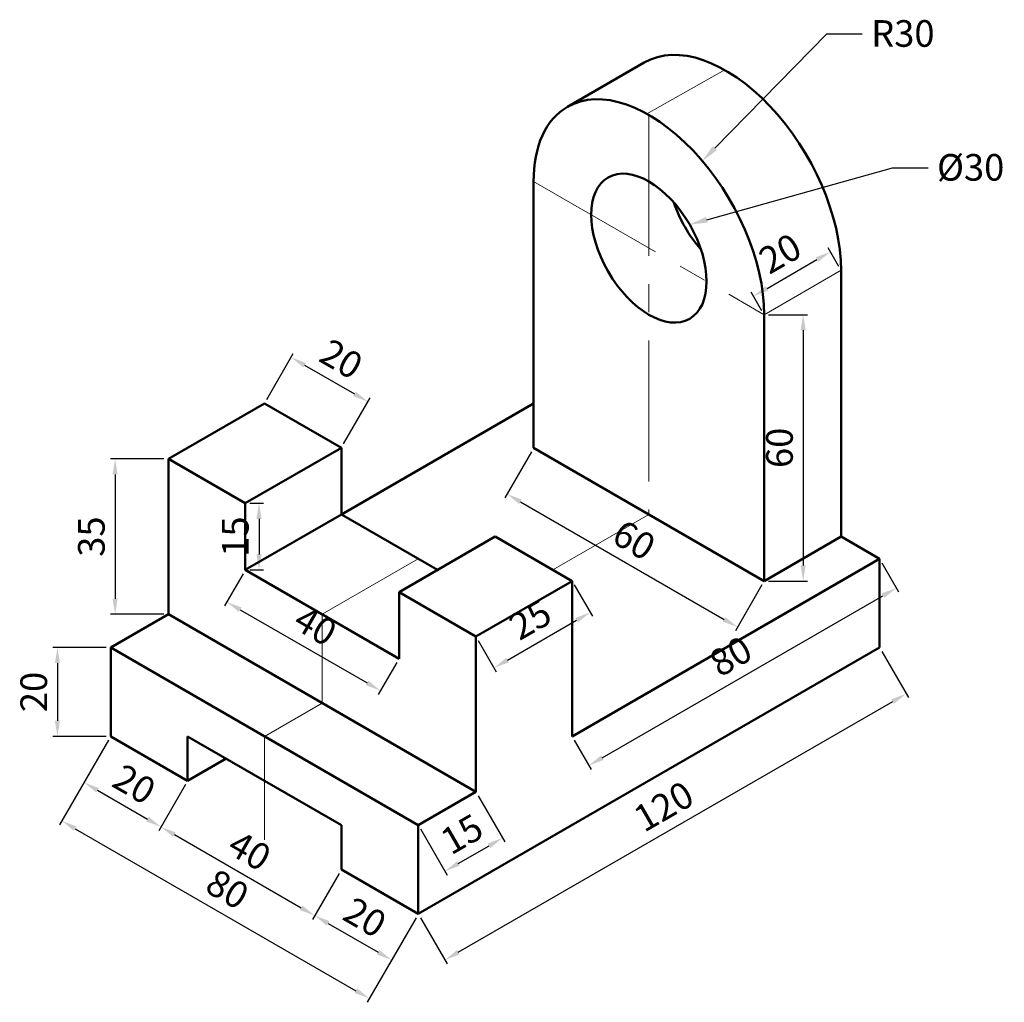
# Model space of a CAD drawing. Units: millimetres. Extents: x 3098 to 3319, y 970 to 1192.
import ezdxf
from ezdxf import colors
from ezdxf.entities.mleader import LeaderData, LeaderLine
from ezdxf.math import Vec2, Vec3

# ---------------------------------------------------------------- set-up
doc = ezdxf.new("R2010")
doc.units = ezdxf.units.MM
doc.linetypes.add('CENTER', pattern=[50.8, 31.75, -6.35, 6.35, -6.35])
for name, color, linetype, lineweight in [('M-CNTR', 1, 'CENTER', 18), ('M-DIMS', 3, 'Continuous', 25), ('M-OUTL', 7, 'Continuous', 50)]:
    doc.layers.add(name, color=color, linetype=linetype, lineweight=lineweight)
doc.styles.get("Standard").update_dxf_attribs({"font": 'arial.ttf'})
doc.dimstyles.new('AM_ISO$0', dxfattribs={"dimtxt": 6, "dimasz": 3.5, "dimexe": 1, "dimexo": 1, "dimgap": 1.5, "dimtad": 1, "dimdsep": 46, "dimtxsty": 'Standard', "dimcen": 0, "dimclrd": 256, "dimclre": 256, "dimclrt": 2, "dimadec": 0, "dimazin": 2, "dimtp": 0.1, "dimtm": 0.1, "dimtfac": 0.71, "dimtmove": 0, "dimatfit": 3, "dimfxl": 1, "dimlwd": -1, "dimlwe": -1, "dimarcsym": 1})

# ---------------------------------------------------------------- blocks, each defined once
blk = doc.blocks.new('*D3')
at = {"layer": 'Defpoints', "color": 0, "transparency": 16777216}
for p in [(3291.25, 1050.05), (3297.25, 1039.66), (3187.33, 990.05)]:
    blk.add_point(p, dxfattribs=at)
at = {"layer": 'M-DIMS', "color": 0, "linetype": 'ByBlock', "transparency": 16777216}
for p, q in [((3291.75, 1049.18), (3297.75, 1038.79)), ((3196.36, 981.41), (3294.22, 1037.91)), ((3187.83, 989.18), (3193.83, 978.79))]:
    blk.add_line(p, q, dxfattribs=at)
at = {"layer": 'M-DIMS', "color": 0, "transparency": 16777216}
for points in [[(3293.93, 1038.41), (3294.51, 1037.4), (3297.25, 1039.66)], [(3196.07, 981.91), (3196.65, 980.9), (3193.33, 979.66)]]:
    blk.add_solid(points, dxfattribs=at)
at = {"layer": 'M-DIMS', "color": 0, "transparency": 16777216, "insert": (3243.01, 1013.61), "char_height": 6, "attachment_point": 5, "rotation": 30}
blk.add_mtext('120', dxfattribs=at)
blk = doc.blocks.new('*D4')
at = {"layer": 'Defpoints', "color": 0, "transparency": 16777216}
for p in [(3291.25, 1070.05), (3295.05, 1063.48), (3221.97, 1030.05)]:
    blk.add_point(p, dxfattribs=at)
at = {"layer": 'M-DIMS', "color": 0, "linetype": 'ByBlock', "transparency": 16777216}
for p, q in [((3291.75, 1069.18), (3295.55, 1062.61)), ((3228.8, 1025.23), (3292.02, 1061.73)), ((3222.47, 1029.18), (3226.27, 1022.61))]:
    blk.add_line(p, q, dxfattribs=at)
at = {"layer": 'M-DIMS', "color": 0, "transparency": 16777216}
for points in [[(3291.72, 1062.24), (3292.31, 1061.23), (3295.05, 1063.48)], [(3228.5, 1025.74), (3229.09, 1024.73), (3225.77, 1023.48)]]:
    blk.add_solid(points, dxfattribs=at)
at = {"layer": 'M-DIMS', "color": 0, "transparency": 16777216, "insert": (3258.12, 1047.43), "char_height": 6, "attachment_point": 5, "rotation": 30}
blk.add_mtext('80', dxfattribs=at)
blk = doc.blocks.new('*D5')
at = {"layer": 'Defpoints', "color": 0, "transparency": 16777216}
for p in [(3221.97, 1065.05), (3226.06, 1057.98), (3200.32, 1052.55)]:
    blk.add_point(p, dxfattribs=at)
at = {"layer": 'M-DIMS', "color": 0, "linetype": 'ByBlock', "transparency": 16777216}
for p, q in [((3222.47, 1064.18), (3226.56, 1057.11)), ((3207.44, 1047.23), (3223.02, 1056.23)), ((3200.82, 1051.68), (3204.9, 1044.61))]:
    blk.add_line(p, q, dxfattribs=at)
at = {"layer": 'M-DIMS', "color": 0, "transparency": 16777216}
for points in [[(3222.73, 1056.73), (3223.32, 1055.72), (3226.06, 1057.98)], [(3207.14, 1047.73), (3207.73, 1046.72), (3204.4, 1045.48)]]:
    blk.add_solid(points, dxfattribs=at)
at = {"layer": 'M-DIMS', "color": 0, "transparency": 16777216, "insert": (3212.95, 1055.68), "char_height": 6, "attachment_point": 5, "rotation": 30}
blk.add_mtext('25', dxfattribs=at)
blk = doc.blocks.new('*D6')
at = {"layer": 'Defpoints', "color": 0, "transparency": 16777216}
for p in [(3131.04, 1092.55), (3119.04, 1057.55), (3131.04, 1057.55)]:
    blk.add_point(p, dxfattribs=at)
at = {"layer": 'M-DIMS', "color": 0, "linetype": 'ByBlock', "transparency": 16777216}
for p, q in [((3130.04, 1092.55), (3118.04, 1092.55)), ((3119.04, 1089.05), (3119.04, 1061.05)), ((3130.04, 1057.55), (3118.04, 1057.55))]:
    blk.add_line(p, q, dxfattribs=at)
at = {"layer": 'M-DIMS', "color": 0, "transparency": 16777216}
for points in [[(3118.46, 1089.05), (3119.62, 1089.05), (3119.04, 1092.55)], [(3118.46, 1061.05), (3119.62, 1061.05), (3119.04, 1057.55)]]:
    blk.add_solid(points, dxfattribs=at)
at = {"layer": 'M-DIMS', "color": 0, "transparency": 16777216, "insert": (3114.47, 1075.05), "char_height": 6, "attachment_point": 5, "rotation": 90}
blk.add_mtext('35', dxfattribs=at)
blk = doc.blocks.new('*D7')
at = {"layer": 'Defpoints', "color": 0, "transparency": 16777216}
for p in [(3118.05, 1050.05), (3106.05, 1030.05), (3118.05, 1030.05)]:
    blk.add_point(p, dxfattribs=at)
at = {"layer": 'M-DIMS', "color": 0, "linetype": 'ByBlock', "transparency": 16777216}
for p, q in [((3117.05, 1050.05), (3105.05, 1050.05)), ((3106.05, 1046.55), (3106.05, 1033.55)), ((3117.05, 1030.05), (3105.05, 1030.05))]:
    blk.add_line(p, q, dxfattribs=at)
at = {"layer": 'M-DIMS', "color": 0, "transparency": 16777216}
for points in [[(3105.47, 1046.55), (3106.63, 1046.55), (3106.05, 1050.05)], [(3105.47, 1033.55), (3106.63, 1033.55), (3106.05, 1030.05)]]:
    blk.add_solid(points, dxfattribs=at)
at = {"layer": 'M-DIMS', "color": 0, "transparency": 16777216, "insert": (3101.49, 1040.05), "char_height": 6, "attachment_point": 5, "rotation": 90}
blk.add_mtext('20', dxfattribs=at)
blk = doc.blocks.new('*D8')
at = {"layer": 'Defpoints', "color": 0, "transparency": 16777216}
for p in [(3118.05, 1030.05), (3135.37, 1020.05), (3129.37, 1009.66)]:
    blk.add_point(p, dxfattribs=at)
at = {"layer": 'M-DIMS', "color": 0, "linetype": 'ByBlock', "transparency": 16777216}
for p, q in [((3117.55, 1029.18), (3111.55, 1018.79)), ((3134.87, 1019.18), (3128.87, 1008.79)), ((3115.08, 1017.91), (3126.34, 1011.41))]:
    blk.add_line(p, q, dxfattribs=at)
at = {"layer": 'M-DIMS', "color": 0, "transparency": 16777216}
for points in [[(3115.37, 1018.41), (3114.79, 1017.4), (3112.05, 1019.66)], [(3126.63, 1011.91), (3126.05, 1010.9), (3129.37, 1009.66)]]:
    blk.add_solid(points, dxfattribs=at)
at = {"layer": 'M-DIMS', "color": 0, "transparency": 16777216, "insert": (3122.99, 1018.61), "char_height": 6, "attachment_point": 5, "rotation": 330}
blk.add_mtext('20', dxfattribs=at)
blk = doc.blocks.new('*D9')
at = {"layer": 'Defpoints', "color": 0, "transparency": 16777216}
for p in [(3135.37, 1020.05), (3170.01, 1000.05), (3164.01, 989.66)]:
    blk.add_point(p, dxfattribs=at)
at = {"layer": 'M-DIMS', "color": 0, "linetype": 'ByBlock', "transparency": 16777216}
for p, q in [((3134.87, 1019.18), (3128.87, 1008.79)), ((3132.4, 1007.91), (3160.98, 991.41)), ((3169.51, 999.18), (3163.51, 988.79))]:
    blk.add_line(p, q, dxfattribs=at)
at = {"layer": 'M-DIMS', "color": 0, "transparency": 16777216}
for points in [[(3132.69, 1008.41), (3132.11, 1007.4), (3129.37, 1009.66)], [(3161.27, 991.91), (3160.69, 990.9), (3164.01, 989.66)]]:
    blk.add_solid(points, dxfattribs=at)
at = {"layer": 'M-DIMS', "color": 0, "transparency": 16777216, "insert": (3148.97, 1003.61), "char_height": 6, "attachment_point": 5, "rotation": 330}
blk.add_mtext('40', dxfattribs=at)
blk = doc.blocks.new('*D10')
at = {"layer": 'Defpoints', "color": 0, "transparency": 16777216}
for p in [(3170.01, 1000.05), (3187.33, 990.05), (3181.33, 979.66)]:
    blk.add_point(p, dxfattribs=at)
at = {"layer": 'M-DIMS', "color": 0, "linetype": 'ByBlock', "transparency": 16777216}
for p, q in [((3169.51, 999.18), (3163.51, 988.79)), ((3167.04, 987.91), (3178.3, 981.41)), ((3186.83, 989.18), (3180.83, 978.79))]:
    blk.add_line(p, q, dxfattribs=at)
at = {"layer": 'M-DIMS', "color": 0, "transparency": 16777216}
for points in [[(3167.33, 988.41), (3166.75, 987.4), (3164.01, 989.66)], [(3178.59, 981.91), (3178.01, 980.9), (3181.33, 979.66)]]:
    blk.add_solid(points, dxfattribs=at)
at = {"layer": 'M-DIMS', "color": 0, "transparency": 16777216, "insert": (3174.95, 988.61), "char_height": 6, "attachment_point": 5, "rotation": 330}
blk.add_mtext('20', dxfattribs=at)
blk = doc.blocks.new('*D11')
at = {"layer": 'Defpoints', "color": 0, "transparency": 16777216}
for p in [(3118.05, 1030.05), (3187.33, 990.05), (3176.33, 971)]:
    blk.add_point(p, dxfattribs=at)
at = {"layer": 'M-DIMS', "color": 0, "linetype": 'ByBlock', "transparency": 16777216}
for p, q in [((3117.55, 1029.18), (3106.55, 1010.13)), ((3110.08, 1009.25), (3173.3, 972.75)), ((3186.83, 989.18), (3175.83, 970.13))]:
    blk.add_line(p, q, dxfattribs=at)
at = {"layer": 'M-DIMS', "color": 0, "transparency": 16777216}
for points in [[(3110.37, 1009.75), (3109.79, 1008.74), (3107.05, 1011)], [(3173.59, 973.25), (3173.01, 972.24), (3176.33, 971)]]:
    blk.add_solid(points, dxfattribs=at)
at = {"layer": 'M-DIMS', "color": 0, "transparency": 16777216, "insert": (3143.97, 994.95), "char_height": 6, "attachment_point": 5, "rotation": 330}
blk.add_mtext('80', dxfattribs=at)
blk = doc.blocks.new('*D12')
at = {"layer": 'Defpoints', "color": 0, "transparency": 16777216}
for p in [(3152.69, 1105.05), (3176.01, 1105.44), (3170.01, 1095.05)]:
    blk.add_point(p, dxfattribs=at)
at = {"layer": 'M-DIMS', "color": 0, "linetype": 'ByBlock', "transparency": 16777216}
for p, q in [((3153.19, 1105.92), (3159.19, 1116.31)), ((3161.72, 1113.69), (3172.98, 1107.19)), ((3170.51, 1095.92), (3176.51, 1106.31))]:
    blk.add_line(p, q, dxfattribs=at)
at = {"layer": 'M-DIMS', "color": 0, "transparency": 16777216}
for points in [[(3162.01, 1114.2), (3161.43, 1113.19), (3158.69, 1115.44)], [(3173.27, 1107.7), (3172.69, 1106.69), (3176.01, 1105.44)]]:
    blk.add_solid(points, dxfattribs=at)
at = {"layer": 'M-DIMS', "color": 0, "transparency": 16777216, "insert": (3169.63, 1114.4), "char_height": 6, "attachment_point": 5, "rotation": 330}
blk.add_mtext('20', dxfattribs=at)
blk = doc.blocks.new('*D13')
at = {"layer": 'Defpoints', "color": 0, "transparency": 16777216}
for p in [(3148.36, 1082.55), (3148.36, 1067.55), (3151.46, 1067.55)]:
    blk.add_point(p, dxfattribs=at)
at = {"layer": 'M-DIMS', "color": 0, "linetype": 'ByBlock', "transparency": 16777216}
for p, q in [((3149.36, 1082.55), (3152.46, 1082.55)), ((3151.46, 1079.05), (3151.46, 1071.05)), ((3149.36, 1067.55), (3152.46, 1067.55))]:
    blk.add_line(p, q, dxfattribs=at)
at = {"layer": 'M-DIMS', "color": 0, "transparency": 16777216}
for points in [[(3150.88, 1079.05), (3152.04, 1079.05), (3151.46, 1082.55)], [(3150.88, 1071.05), (3152.04, 1071.05), (3151.46, 1067.55)]]:
    blk.add_solid(points, dxfattribs=at)
at = {"layer": 'M-DIMS', "color": 0, "transparency": 16777216, "insert": (3146.9, 1075.05), "char_height": 6, "attachment_point": 5, "rotation": 90}
blk.add_mtext('15', dxfattribs=at)
blk = doc.blocks.new('*D14')
at = {"layer": 'Defpoints', "color": 0, "transparency": 16777216}
for p in [(3148.36, 1067.55), (3183, 1047.55), (3178.84, 1040.34)]:
    blk.add_point(p, dxfattribs=at)
at = {"layer": 'M-DIMS', "color": 0, "linetype": 'ByBlock', "transparency": 16777216}
for p, q in [((3147.86, 1066.68), (3143.7, 1059.47)), ((3147.23, 1058.59), (3175.81, 1042.09)), ((3182.5, 1046.68), (3178.34, 1039.47))]:
    blk.add_line(p, q, dxfattribs=at)
at = {"layer": 'M-DIMS', "color": 0, "transparency": 16777216}
for points in [[(3147.52, 1059.09), (3146.93, 1058.08), (3144.2, 1060.34)], [(3176.1, 1042.59), (3175.51, 1041.58), (3178.84, 1040.34)]]:
    blk.add_solid(points, dxfattribs=at)
at = {"layer": 'M-DIMS', "color": 0, "transparency": 16777216, "insert": (3163.8, 1054.29), "char_height": 6, "attachment_point": 5, "rotation": 330}
blk.add_mtext('40', dxfattribs=at)
blk = doc.blocks.new('*D15')
at = {"layer": 'Defpoints', "color": 0, "transparency": 16777216}
for p in [(3265.27, 1125.05), (3265.27, 1065.05), (3274.04, 1065.05)]:
    blk.add_point(p, dxfattribs=at)
at = {"layer": 'M-DIMS', "color": 0, "linetype": 'ByBlock', "transparency": 16777216}
for p, q in [((3266.27, 1125.05), (3275.04, 1125.05)), ((3274.04, 1121.55), (3274.04, 1068.55)), ((3266.27, 1065.05), (3275.04, 1065.05))]:
    blk.add_line(p, q, dxfattribs=at)
at = {"layer": 'M-DIMS', "color": 0, "transparency": 16777216}
for points in [[(3273.46, 1121.55), (3274.62, 1121.55), (3274.04, 1125.05)], [(3273.46, 1068.55), (3274.62, 1068.55), (3274.04, 1065.05)]]:
    blk.add_solid(points, dxfattribs=at)
at = {"layer": 'M-DIMS', "color": 0, "transparency": 16777216, "insert": (3269.48, 1095.05), "char_height": 6, "attachment_point": 5, "rotation": 90}
blk.add_mtext('60', dxfattribs=at)
blk = doc.blocks.new('*D16')
at = {"layer": 'Defpoints', "color": 0, "transparency": 16777216}
for p in [(3280.19, 1139.22), (3282.59, 1135.05), (3265.27, 1125.05)]:
    blk.add_point(p, dxfattribs=at)
at = {"layer": 'M-DIMS', "color": 0, "linetype": 'ByBlock', "transparency": 16777216}
for p, q in [((3282.09, 1135.92), (3279.69, 1140.09)), ((3265.9, 1130.97), (3277.15, 1137.47)), ((3264.77, 1125.92), (3262.36, 1130.09))]:
    blk.add_line(p, q, dxfattribs=at)
at = {"layer": 'M-DIMS', "color": 0, "transparency": 16777216}
for points in [[(3276.86, 1137.98), (3277.45, 1136.97), (3280.19, 1139.22)], [(3265.6, 1131.48), (3266.19, 1130.47), (3262.86, 1129.22)]]:
    blk.add_solid(points, dxfattribs=at)
at = {"layer": 'M-DIMS', "color": 0, "transparency": 16777216, "insert": (3269.24, 1138.18), "char_height": 6, "attachment_point": 5, "rotation": 30}
blk.add_mtext('20', dxfattribs=at)
blk = doc.blocks.new('*D17')
at = {"layer": 'Defpoints', "color": 0, "transparency": 16777216}
for p in [(3213.31, 1095.05), (3265.27, 1065.05), (3259.27, 1054.66)]:
    blk.add_point(p, dxfattribs=at)
at = {"layer": 'M-DIMS', "color": 0, "linetype": 'ByBlock', "transparency": 16777216}
for p, q in [((3212.81, 1094.18), (3206.81, 1083.79)), ((3210.34, 1082.91), (3256.24, 1056.41)), ((3264.77, 1064.18), (3258.77, 1053.79))]:
    blk.add_line(p, q, dxfattribs=at)
at = {"layer": 'M-DIMS', "color": 0, "transparency": 16777216}
for points in [[(3210.63, 1083.41), (3210.05, 1082.4), (3207.31, 1084.66)], [(3256.53, 1056.91), (3255.95, 1055.9), (3259.27, 1054.66)]]:
    blk.add_solid(points, dxfattribs=at)
at = {"layer": 'M-DIMS', "color": 0, "transparency": 16777216, "insert": (3235.57, 1073.61), "char_height": 6, "attachment_point": 5, "rotation": 330}
blk.add_mtext('60', dxfattribs=at)
blk = doc.blocks.new('*D18')
at = {"layer": 'Defpoints', "color": 0, "transparency": 16777216}
for p in [(3200.32, 1017.55), (3187.33, 1010.05), (3206.32, 1007.16)]:
    blk.add_point(p, dxfattribs=at)
at = {"layer": 'M-DIMS', "color": 0, "linetype": 'ByBlock', "transparency": 16777216}
for p, q in [((3200.82, 1016.68), (3206.82, 1006.29)), ((3187.83, 1009.18), (3193.83, 998.79)), ((3196.36, 1001.41), (3203.29, 1005.41))]:
    blk.add_line(p, q, dxfattribs=at)
at = {"layer": 'M-DIMS', "color": 0, "transparency": 16777216}
for points in [[(3203, 1005.91), (3203.58, 1004.9), (3206.32, 1007.16)], [(3196.07, 1001.91), (3196.65, 1000.9), (3193.33, 999.66)]]:
    blk.add_solid(points, dxfattribs=at)
at = {"layer": 'M-DIMS', "color": 0, "transparency": 16777216, "insert": (3197.54, 1007.36), "char_height": 6, "attachment_point": 5, "rotation": 30}
blk.add_mtext('15', dxfattribs=at)

msp = doc.modelspace()

# ---------------------------------------------------------------- linework, layer by layer
at = {"layer": 'M-CNTR'}
for p, q in [((3238.806, 1170.326), (3256.374, 1180.187)), ((3239.293, 1170.051), (3239.293, 1080.051)), ((3213.312, 1155.051), (3265.273, 1125.051)), ((3265.273, 1125.051), (3282.594, 1135.051)), ((3239.293, 1080.051), (3217.642, 1067.551)), ((3165.681, 1057.551), (3187.331, 1070.051)), ((3165.681, 1037.551), (3165.681, 1057.551)), ((3165.681, 1037.551), (3152.69, 1030.051)), ((3152.69, 1030.051), (3152.69, 1006.719))]:
    msp.add_line(p, q, dxfattribs=at)
at = {"layer": 'M-OUTL'}
for p, q in [((3238.242, 1181.87), (3220.922, 1171.87)), ((3213.312, 1095.051), (3213.312, 1155.051)), ((3282.594, 1075.051), (3282.594, 1135.051)), ((3265.273, 1065.051), (3265.273, 1125.051)), ((3131.04, 1092.551), (3152.69, 1105.051)), ((3170.011, 1095.051), (3152.69, 1105.051)), ((3213.312, 1105.051), (3170.011, 1080.051)), ((3148.36, 1082.551), (3170.011, 1095.051)), ((3170.011, 1095.051), (3170.011, 1080.051)), ((3265.273, 1065.051), (3213.312, 1095.051)), ((3131.04, 1057.551), (3131.04, 1092.551)), ((3131.04, 1092.551), (3148.36, 1082.551)), ((3148.36, 1082.551), (3131.04, 1092.551)), ((3148.36, 1082.551), (3148.36, 1067.551)), ((3148.36, 1067.551), (3170.011, 1080.051)), ((3170.011, 1080.051), (3191.661, 1067.551)), ((3239.293, 1080.051), (3265.273, 1065.051)), ((3183.001, 1062.551), (3204.652, 1075.051)), ((3221.972, 1065.051), (3204.652, 1075.051)), ((3265.273, 1065.051), (3282.594, 1075.051)), ((3291.254, 1070.051), (3282.594, 1075.051)), ((3291.254, 1070.051), (3221.972, 1030.051)), ((3291.254, 1050.051), (3291.254, 1070.051)), ((3148.36, 1067.551), (3183.001, 1047.551)), ((3221.972, 1065.051), (3200.322, 1052.551)), ((3221.972, 1030.051), (3221.972, 1065.051)), ((3200.322, 1052.551), (3183.001, 1062.551)), ((3183.001, 1047.551), (3183.001, 1062.551)), ((3131.04, 1057.551), (3118.049, 1050.051)), ((3200.322, 1017.551), (3131.04, 1057.551)), ((3200.322, 1052.551), (3200.322, 1017.551)), ((3187.331, 1010.051), (3118.049, 1050.051)), ((3118.049, 1050.051), (3118.049, 1030.051)), ((3187.331, 990.051), (3291.254, 1050.051)), ((3118.049, 1030.051), (3135.37, 1020.051)), ((3135.37, 1020.051), (3135.37, 1030.051)), ((3135.37, 1030.051), (3170.011, 1010.051)), ((3135.37, 1020.051), (3144.03, 1025.051)), ((3200.322, 1017.551), (3187.331, 1010.051)), ((3170.011, 1010.051), (3170.011, 1000.051)), ((3187.331, 1010.051), (3187.331, 990.051)), ((3170.011, 1000.051), (3187.331, 990.051))]:
    msp.add_line(p, q, dxfattribs=at)
for centre, major_axis, start_param, end_param in [((3256.613, 1150.051), (18.371, -31.82), 7.0685835, 9.424778), ((3239.293, 1140.051), (18.371, -31.82), 0.7853982, 3.1415927), ((3239.293, 1140.051), (18.371, -31.82), 3.1415927, 3.9269908), ((3256.613, 1150.051), (9.186, -15.91), 4.3725521, 5.0522259)]:
    msp.add_ellipse(centre, major_axis=major_axis, ratio=0.5773503, start_param=start_param, end_param=end_param, dxfattribs=at)
msp.add_ellipse((3239.293, 1140.051), major_axis=(9.186, -15.91), ratio=0.5773503, dxfattribs=at)

# ---------------------------------------------------------------- dimensions: what is measured, and where the dimension line sits
at = {"layer": 'M-DIMS'}
for p1, p2, distance, override, picture, middle in [((3265.273, 1125.051), (3282.594, 1135.051), 4.818, {"dimclrd": 0, "dimclre": 0, "dimclrt": 0}, '*D16', (3269.243, 1138.175)), ((3265.273, 1125.051), (3265.273, 1065.051), 8.768, {"dimclrd": 0, "dimclre": 0, "dimclrt": 0}, '*D15', (3269.478, 1095.051)), ((3152.69, 1105.051), (3170.011, 1095.051), 12, {"dimclrd": 0, "dimclre": 0, "dimclrt": 0}, '*D12', (3169.632, 1114.395)), ((3213.312, 1095.051), (3265.273, 1065.051), -12, {"dimclrd": 0, "dimclre": 0, "dimclrt": 0}, '*D17', (3235.574, 1073.61)), ((3131.04, 1092.551), (3131.04, 1057.551), -12, {"dimclrd": 0, "dimclre": 0, "dimclrt": 0}, '*D6', (3114.474, 1075.051)), ((3148.36, 1082.551), (3148.36, 1067.551), 3.099, {"dimclrd": 0, "dimclre": 0, "dimclrt": 0}, '*D13', (3146.896, 1075.051)), ((3221.972, 1030.051), (3291.254, 1070.051), -7.586, {"dimclrd": 0, "dimclre": 0, "dimclrt": 0}, '*D4', (3258.125, 1047.433)), ((3148.36, 1067.551), (3183.001, 1047.551), -8.329, {"dimclrd": 0, "dimclre": 0, "dimclrt": 0}, '*D14', (3163.798, 1054.289)), ((3200.322, 1052.551), (3221.972, 1065.051), -8.166, {"dimclrd": 0, "dimclre": 0, "dimclrt": 0}, '*D5', (3212.948, 1055.681)), ((3118.049, 1050.051), (3118.049, 1030.051), -12, {"dimclrd": 0, "dimclre": 0, "dimclrt": 0}, '*D7', (3101.486, 1040.051)), ((3187.331, 990.051), (3291.254, 1050.051), -12, {"dimpost": '', "dimclrd": 0, "dimclre": 0, "dimclrt": 0}, '*D3', (3243.011, 1013.61)), ((3118.049, 1030.051), (3187.331, 990.051), -22, {"dimclrd": 0, "dimclre": 0, "dimclrt": 0}, '*D11', (3143.972, 994.95)), ((3118.049, 1030.051), (3135.37, 1020.051), -12, {"dimclrd": 0, "dimclre": 0, "dimclrt": 0}, '*D8', (3122.991, 1018.61)), ((3135.37, 1020.051), (3170.011, 1000.051), -12, {"dimclrd": 0, "dimclre": 0, "dimclrt": 0}, '*D9', (3148.972, 1003.61)), ((3187.331, 1010.051), (3200.322, 1017.551), -12, {"dimclrd": 0, "dimclre": 0, "dimclrt": 0}, '*D18', (3197.545, 1007.36)), ((3170.011, 1000.051), (3187.331, 990.051), -12, {"dimclrd": 0, "dimclre": 0, "dimclrt": 0}, '*D10', (3174.953, 988.61))]:
    dim = msp.add_aligned_dim(p1=p1, p2=p2, distance=distance, dimstyle='AM_ISO$0', override=override, dxfattribs=at)
    dim.commit()
    dim.dimension.update_dxf_attribs({"geometry": picture, "text_midpoint": middle})

# ---------------------------------------------------------------- leaders
ml = msp.add_multileader_mtext('Standard', dxfattribs=at)
ml.set_content('{\\C2;R30}', color=256)
ml.set_leader_properties()
ml.build(insert=Vec2(0, 0))
ctx = ml.context
ctx.base_point, ctx.char_height, ctx.plane_origin = Vec3(3287.362, 1188.352), 6, Vec3(3251.326, 1159.691)
notes = []
notes.append((ctx, [(0, (1, 1, 0), (3279.362, 1188.352), (1, 0), 8, [(0, [(3251.326, 1159.691)], 0, [])])]))
ctx.mtext.insert, ctx.mtext.flow_direction = Vec3(3289.362, 1191.405), 5
ml = msp.add_multileader_mtext('Standard', dxfattribs=at)
ml.set_content('{\\C2;%%C30}', color=256)
ml.set_leader_properties()
ml.build(insert=Vec2(0, 0))
ctx = ml.context
ctx.base_point, ctx.char_height, ctx.plane_origin = Vec3(3302.198, 1158.126), 6, Vec3(3248.478, 1145.354)
notes.append((ctx, [(0, (1, 1, 0), (3294.198, 1158.126), (1, 0), 8, [(0, [(3248.478, 1145.354)], 0, [])])]))
ctx.mtext.insert, ctx.mtext.flow_direction = Vec3(3304.198, 1161.247), 5
for ctx, leaders in notes:
    for number, flags, end, landing, length, lines in leaders:
        leader = LeaderData()
        leader.index, (leader.has_last_leader_line, leader.has_dogleg_vector, leader.attachment_direction) = number, flags
        leader.last_leader_point, leader.dogleg_vector, leader.dogleg_length = Vec3(end), Vec3(landing), length
        for number, points, colour, breaks in lines:
            line = LeaderLine()
            line.index, line.vertices, line.color, line.breaks = number, Vec3.list(points), colors.encode_raw_color(colour), breaks
            leader.lines.append(line)
        ctx.leaders.append(leader)

doc.saveas('drawing.dxf')
